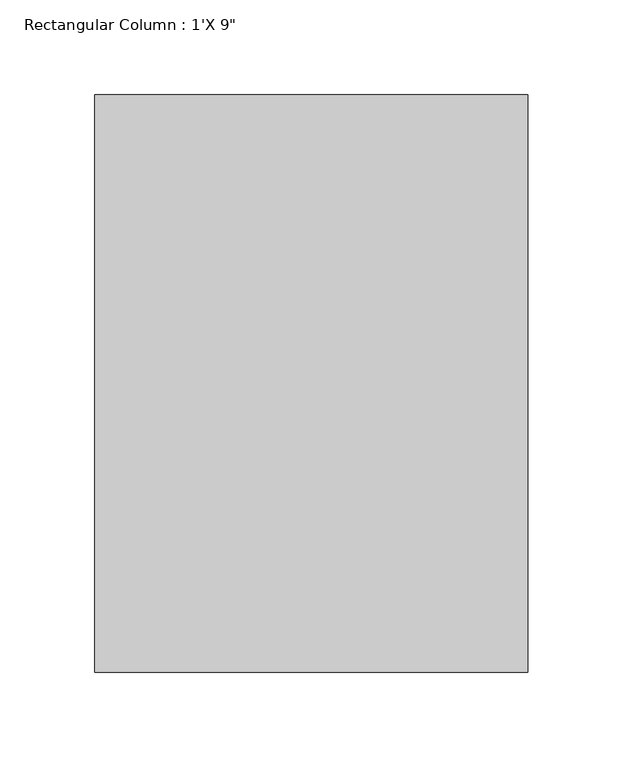
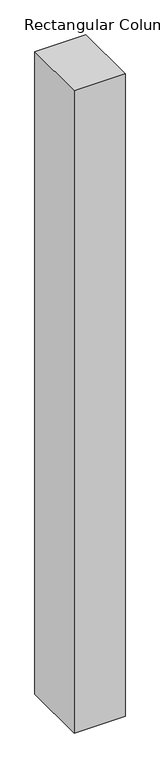
"""IFC4 building model written with IfcOpenShell, lengths in millimetres: column geometry."""

from ifc_helpers import new_model, si_unit, frame, origin, place, context, project, spatial, polyline, outline, extrude, source, transform, mapped, element, save


def column_69e4a381(model_context):
    return source(origin(), model_context, "Body", "SweptSolid", [
        extrude(outline(polyline([(114.3, 152.4), (114.3, -152.4), (-114.3, -152.4), (-114.3, 152.4), (114.3, 152.4)])), frame((0.0, 0.0, 35204.4), z_axis=(0.0, 0.0, 1.0), x_axis=(1.0, 0.0, 0.0)), (0.0, 0.0, 1.0), 3048.0),
    ])


if __name__ == "__main__":
    model = new_model("IFC4")
    model_context = context("Model", 3, world=origin())
    ifc_project = project(units=[si_unit("LENGTHUNIT", "METRE", prefix="MILLI")], contexts=[model_context])
    site = spatial("IfcSite", under=ifc_project)
    building = spatial("IfcBuilding", under=site)
    placement = place(None, origin())
    column_shape = column_69e4a381(model_context)
    element("IfcColumn", 1, ObjectType="Rectangular Column : 1'X 9\"", at=placement, inside=building, context=model_context, shape_type="MappedRepresentation", body=[
        mapped(column_shape, transform((0.0, 0.0, 0.0), x_axis=(1.0, 0.0, 0.0), y_axis=(0.0, 1.0, 0.0), z_axis=(0.0, 0.0, 1.0))),
    ])
    save(model, "model.ifc")

# Revit data of these elements
# Type "Rectangular Column : 1'X 9\""
#   Assembly Code = "B1010200"
#   Depth = 1' - 0"
#   Offset Base = 0' - 0"
#   Offset Top = 0' - 0"
#   Width = 0' - 9"
#   Material = none
